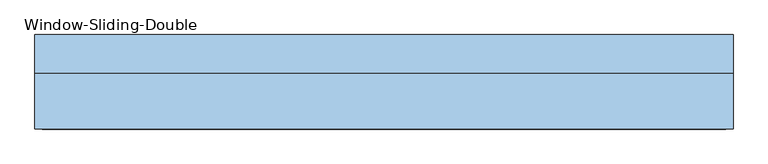
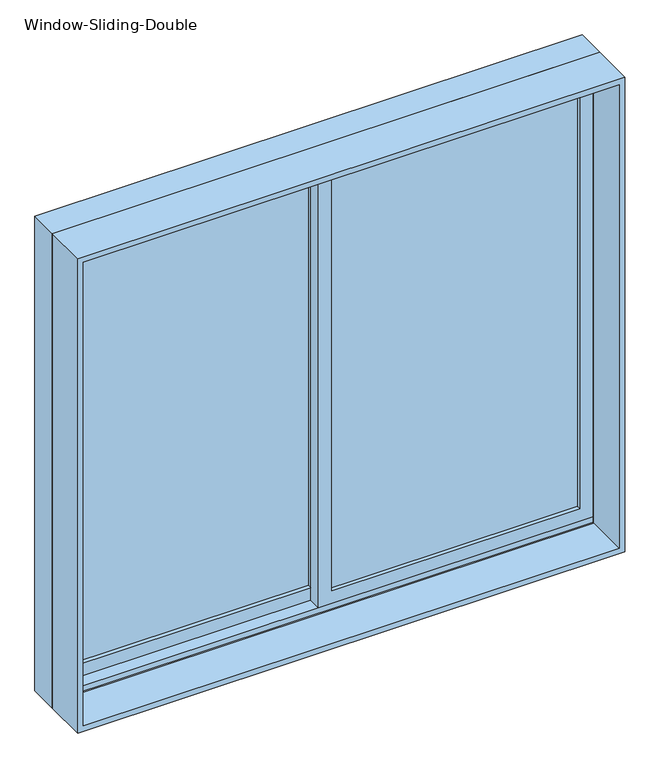
"""IFC4 building model written with IfcOpenShell, lengths in millimetres: window geometry, Window-Sliding-Double."""

from ifc_helpers import new_model, si_unit, frame, origin, place, context, project, spatial, polyline, outline, extrude, faceted_brep, source, transform, mapped, element, save


def window_sliding_double_89c6b595(model_context):
    return source(origin(), model_context, "Body", "SolidModel", [
        extrude(outline(polyline([(952.5, 895.35), (2571.75, 895.35), (2571.75, -22.225), (952.5, -22.225), (952.5, 895.35)]), holes=[polyline([(996.95, 22.225), (2527.3, 22.225), (2527.3, 850.9), (996.95, 850.9), (996.95, 22.225)])]), frame((0.0, 34.29, 0.0), z_axis=(0.0, 1.0, 0.0), x_axis=(0.0, 0.0, 1.0)), (0.0, 0.0, 1.0), 44.45),
        extrude(outline(polyline([(933.45, -895.35), (933.45, 22.225), (2571.75, 22.225), (2571.75, -895.35), (933.45, -895.35)]), holes=[polyline([(2527.3, -22.225), (996.95, -22.225), (996.95, -850.9), (2527.3, -850.9), (2527.3, -22.225)])]), frame((0.0, 78.74, 0.0), z_axis=(0.0, 1.0, 0.0), x_axis=(0.0, 0.0, 1.0)), (0.0, 0.0, 1.0), 44.45),
        extrude(outline(polyline([(-22.225, 110.49), (-22.225, 104.14), (-850.9, 104.14), (-850.9, 110.49), (-22.225, 110.49)])), frame((0.0, 0.0, 996.95), z_axis=(0.0, 0.0, 1.0), x_axis=(1.0, 0.0, 0.0)), (0.0, 0.0, 1.0), 1530.35),
        extrude(outline(polyline([(-22.225, 97.79), (-22.225, 91.44), (-850.9, 91.44), (-850.9, 97.79), (-22.225, 97.79)])), frame((0.0, 0.0, 996.95), z_axis=(0.0, 0.0, 1.0), x_axis=(1.0, 0.0, 0.0)), (0.0, 0.0, 1.0), 1530.35),
        extrude(outline(polyline([(850.9, 66.04), (850.9, 59.69), (22.225, 59.69), (22.225, 66.04), (850.9, 66.04)])), frame((0.0, 0.0, 996.95), z_axis=(0.0, 0.0, 1.0), x_axis=(1.0, 0.0, 0.0)), (0.0, 0.0, 1.0), 1530.35),
        extrude(outline(polyline([(850.9, 53.34), (850.9, 46.99), (22.225, 46.99), (22.225, 53.34), (850.9, 53.34)])), frame((0.0, 0.0, 996.95), z_axis=(0.0, 0.0, 1.0), x_axis=(1.0, 0.0, 0.0)), (0.0, 0.0, 1.0), 1530.35),
        extrude(outline(polyline([(2590.8, -914.4), (914.4, -914.4), (914.4, 914.4), (2590.8, 914.4), (2590.8, -914.4)]), holes=[polyline([(2571.75, 895.35), (933.45, 895.35), (933.45, -895.35), (2571.75, -895.35), (2571.75, 895.35)])]), frame((0.0, -118.11, 0.0), z_axis=(0.0, 1.0, 0.0), x_axis=(0.0, 0.0, 1.0)), (0.0, 0.0, 1.0), 146.05),
        faceted_brep([(-914.4, 27.94, 914.4), (-914.4, 129.54, 914.4), (914.4, 129.54, 914.4), (914.4, 27.94, 914.4), (-873.4778905, 129.54, 2549.8778905), (-873.4778905, 123.19, 2549.8778905), (-873.4778905, 123.19, 933.45), (-873.4778905, 129.54, 933.45), (873.4778905, 123.19, 2549.8778905), (873.4778905, 123.19, 933.45), (895.35, 123.19, 933.45), (895.35, 123.19, 2571.75), (-895.35, 123.19, 2571.75), (-895.35, 123.19, 933.45), (-895.35, 27.94, 2571.75), (-895.35, 27.94, 933.45), (-895.35, 34.29, 933.45), (-895.35, 34.29, 952.5), (-895.35, 78.74, 952.5), (-895.35, 78.74, 933.45), (914.4, 27.94, 2590.8), (-914.4, 27.94, 2590.8), (895.35, 27.94, 2571.75), (895.35, 27.94, 933.45), (-914.4, 129.54, 2590.8), (914.4, 129.54, 2590.8), (873.4778905, 129.54, 933.45), (873.4778905, 129.54, 2549.8778905), (895.35, 78.74, 933.45), (895.35, 78.74, 952.5), (895.35, 34.29, 952.5), (895.35, 34.29, 933.45)], [[[0, 1, 2, 3]], [[4, 5, 6, 7]], [[5, 8, 9, 10, 11, 12, 13, 6]], [[12, 14, 15, 16, 17, 18, 19, 13]], [[0, 3, 20, 21], [22, 23, 15, 14]], [[24, 1, 0, 21]], [[2, 1, 24, 25], [4, 7, 26, 27]], [[5, 4, 27, 8]], [[12, 11, 22, 14]], [[21, 20, 25, 24]], [[8, 27, 26, 9]], [[22, 11, 10, 28, 29, 30, 31, 23]], [[20, 3, 2, 25]], [[26, 7, 6, 13, 19, 28, 10, 9]], [[28, 19, 18, 29]], [[29, 18, 17, 30]], [[30, 17, 16, 31]], [[15, 23, 31, 16]]]),
    ])


if __name__ == "__main__":
    model = new_model("IFC4")
    model_context = context("Model", 3, world=origin())
    ifc_project = project(units=[si_unit("LENGTHUNIT", "METRE", prefix="MILLI")], contexts=[model_context])
    site = spatial("IfcSite", under=ifc_project)
    building = spatial("IfcBuilding", under=site)
    placement = place(None, origin())
    window_sliding_double_shape = window_sliding_double_89c6b595(model_context)
    element("IfcWindow", 1, ObjectType="Window-Sliding-Double", at=placement, inside=building, context=model_context, shape_type="MappedRepresentation", body=[
        mapped(window_sliding_double_shape, transform((0.0, 0.0, 0.0), x_axis=(1.0, 0.0, 0.0), y_axis=(0.0, 1.0, 0.0), z_axis=(0.0, 0.0, 1.0))),
    ])
    save(model, "model.ifc")

# Revit data of these elements
# Type "Window-Sliding-Double"
#   Type Mark = "19"
#   Fire Rating = "0.5h"
#   Assembly Code = "B2020100"
#   Analytic Construction = "Double glazing - domestic"
#   Window Inset [instance default] = 0' - 0"
#   Wall Thickness [instance default] = 0' - 6"
#   Visual Light Transmittance = 0.81
#   Thermal Resistance (R) = 1.8146 (h·ft²·°F)/BTU
#   Solar Heat Gain Coefficient = 0.76
#   Muntin Width = 2' - 8 5/8"
#   Muntin Height = 5' - 0 1/4"
#   Interior Wall Closure [instance default] = 0' - 2 3/4"
#   Heat Transfer Coefficient (U) = 0.5511 BTU/(h·ft²·°F)
#   Frame Extension [instance default] = 0' - 0 1/4"
#   Exterior Wall Closure [instance default] = 0' - 1 1/4"
#   Rough Width = 6' - 0 1/2"
#   Rough Height = 5' - 6 1/2"
#   Height = 5' - 6"
#   Extension Jamb [instance default] = 0' - 2 3/4"
#   Default Sill Height = 3' - 0"
#   Width = 6' - 0"
#   Interior Trim Visibility [instance default] = yes
#   Indicator Visibility [instance default] = yes
#   Exterior Trim Visibility [instance default] = yes
#   Muntin Visibility = yes
#   Extension Jamb Visibility [instance default] = yes
#   Muntin Pattern = Muntin Pattern_2x2 : Muntin Pattern_2x2
#   Interior Trim Material = Wood - Stained
#   Interior Trim = Trim-Window-Interior-Flat : Picture Frame
#   Interior Frame Material = Wood - Stained
#   Glass Panel Material = Glass
#   Exterior Trim Material = Clad - White
#   Exterior Trim = Trim-Window-Exterior-Flat : with Sill
#   Exterior Frame Material = Clad - White
#   Wall Closure = (empty or 0)
# Element 1 (IfcWindow, "Window-Sliding-Double")
#   Wall Thickness = 0' - 9"
#   Extension Jamb = 0' - 5 3/4"
#   Materials on its faces: "Wood - Stained", "Glass", "Clad - White"
# Materials
#   "Wood - Stained": class "Wood", colour RGB 224 178 126, transparency 0, Cost = 0
#   "Glass": class "Glass", colour RGB 0 128 192, transparency 0.75, Description = "Soda Lime Glass", Cost = 0
#   "Clad - White": class "Wood", colour RGB 242 242 238, transparency 0, Cost = 0
